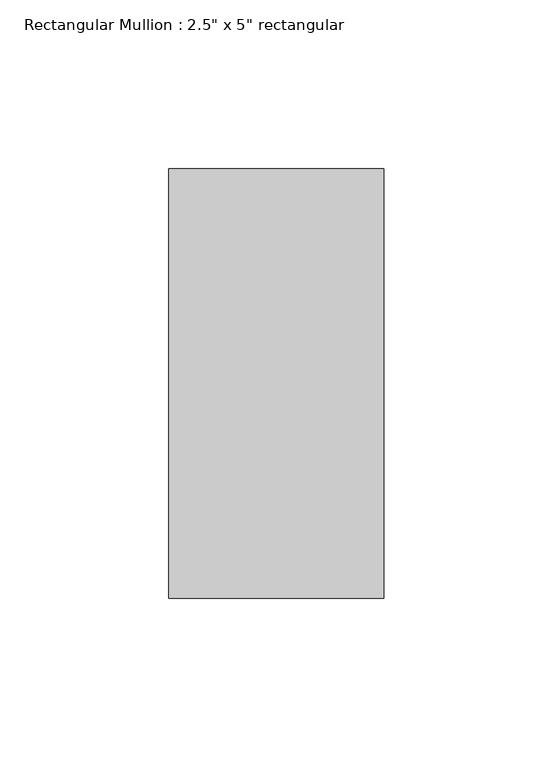
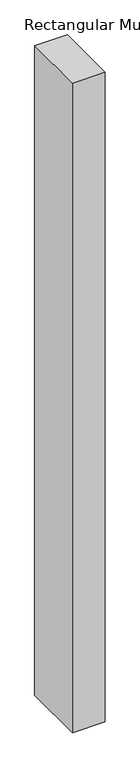
"""IFC4 building model written with IfcOpenShell, lengths in millimetres: member geometry."""

from ifc_helpers import new_model, si_unit, frame, origin, place, context, project, spatial, polyline, outline, extrude, source, transform, mapped, element, save


def member_6e705821(model_context):
    return source(origin(), model_context, "Body", "SweptSolid", [
        extrude(outline(polyline([(0.0, 63.5), (0.0, -63.5), (-63.5, -63.5), (-63.5, 63.5), (0.0, 63.5)])), frame((0.0, 0.0, -1335.6166668), z_axis=(0.0, 0.0, 1.0), x_axis=(1.0, 0.0, 0.0)), (0.0, 0.0, 1.0), 1335.6166668),
    ])


if __name__ == "__main__":
    model = new_model("IFC4")
    model_context = context("Model", 3, world=origin())
    ifc_project = project(units=[si_unit("LENGTHUNIT", "METRE", prefix="MILLI")], contexts=[model_context])
    site = spatial("IfcSite", under=ifc_project)
    building = spatial("IfcBuilding", under=site)
    placement = place(None, origin())
    member_shape = member_6e705821(model_context)
    element("IfcMember", 1, ObjectType="Rectangular Mullion : 2.5\" x 5\" rectangular", at=placement, inside=building, context=model_context, shape_type="MappedRepresentation", body=[
        mapped(member_shape, transform((0.0, 0.0, 0.0), x_axis=(1.0, 0.0, 0.0), y_axis=(0.0, 1.0, 0.0), z_axis=(0.0, 0.0, 1.0))),
    ])
    save(model, "model.ifc")

# Revit data of these elements
# Type "Rectangular Mullion : 2.5\" x 5\" rectangular"
#   built-in parameter 1007304 = 0.416667 (stored number, unit not read)
#   built-in parameter 1007301 = 0.104167 (stored number, unit not read)
#   built-in parameter 1007300 = 0.104167 (stored number, unit not read)
# Element 1 (IfcMember, "Rectangular Mullion : 2.5\" x 5\" rectangular")
#   Materials on its faces: "Aluminum"
# Materials
#   "Aluminum": class "Metal", colour RGB 247 247 247, transparency 0, Description = "Aluminum 6061", Cost = 0
